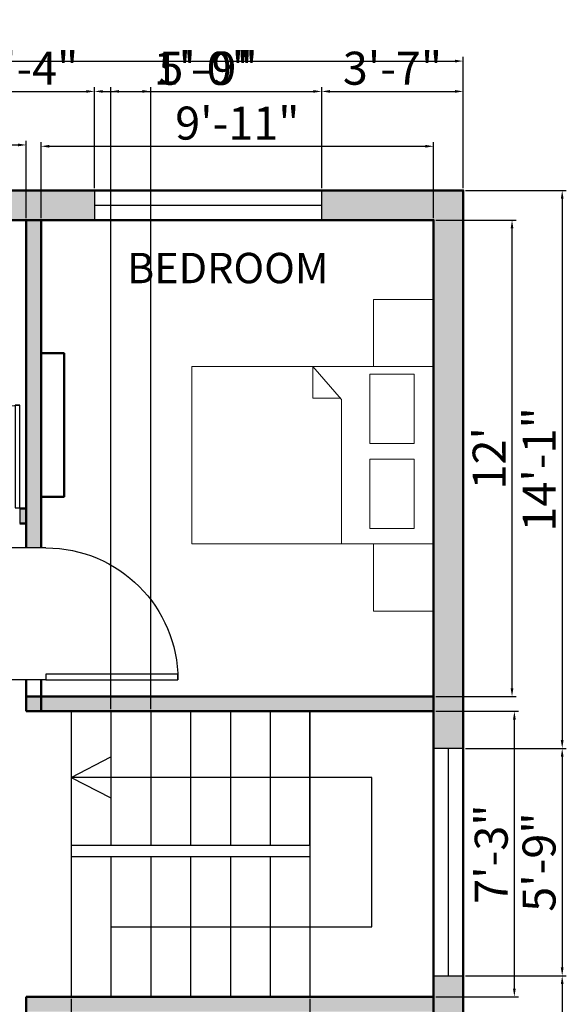
# Model space of a CAD drawing. Units: inches. Extents: x 1344 to 2521, y 3236 to 4924.
# Tile 3 of 14: x 1639 to 1805, y 3517 to 3815. Entities that reach past the tile are written whole.
import ezdxf

# ---------------------------------------------------------------- set-up
doc = ezdxf.new("R2010")
doc.units = ezdxf.units.IN
for name, color, linetype, lineweight in [('A-ANNO-DIMS', 2, 'Continuous', 18), ('A-AREA-IDEN', 3, 'Continuous', 18), ('A-DOOR', 50, 'Continuous', 25), ('A-FLOR-STRS', 7, 'Continuous', 25), ('A-FURN', 130, 'Continuous', 18), ('A-GLAZ', 150, 'Continuous', 25), ('A-WALL', 31, 'Continuous', 50), ('A-WALL-PATT', 8, 'Continuous', 13)]:
    doc.layers.add(name, color=color, linetype=linetype, lineweight=lineweight)
doc.styles.get("Standard").update_dxf_attribs({"font": 'arial.ttf'})
doc.dimstyles.new('ISO-25', dxfattribs={"dimtxt": 10, "dimasz": 2.5, "dimexe": 1.25, "dimexo": 0.625, "dimtad": 1, "dimdec": 0, "dimlunit": 4, "dimtxsty": 'Standard', "dimcen": 2.5, "dimadec": 0, "dimazin": 0, "dimtfac": 1, "dimtdec": 0, "dimtmove": 0, "dimatfit": 3, "dimfxl": 1, "dimarcsym": 0})

# ---------------------------------------------------------------- blocks, each defined once
blk = doc.blocks.new('*U2')
for p, q in [((0, 0), (0, -6)), ((40, 0), (40, -6))]:
    blk.add_line(p, q)
blk.add_lwpolyline([(0, 0), (0, 40), (1.75, 40), (1.75, 0)], close=True)
blk.add_arc((0, 0), 40, 0, 90)
blk = doc.blocks.new('*D32')
at = {"layer": 'A-ANNO-DIMS', "color": 0, "lineweight": -2, "transparency": 16777216}
for p, q in [((1413.52, 3764.06), (1413.52, 3803.88)), ((1773.52, 3764.06), (1773.52, 3803.88)), ((1416.02, 3802.63), (1771.02, 3802.63))]:
    blk.add_line(p, q, dxfattribs=at)
at = {"layer": 'A-ANNO-DIMS', "color": 0, "lineweight": 100, "transparency": 16777216}
for points in [[(1416.02, 3803.04), (1416.02, 3802.21), (1413.52, 3802.63)], [(1771.02, 3803.04), (1771.02, 3802.21), (1773.52, 3802.63)]]:
    blk.add_solid(points, dxfattribs=at)
at = {"layer": 'Defpoints', "color": 0, "lineweight": 100, "transparency": 16777216}
for p in [(1773.52, 3802.63), (1413.52, 3763.43), (1773.52, 3763.43)]:
    blk.add_point(p, dxfattribs=at)
at = {"layer": 'A-ANNO-DIMS', "color": 0, "transparency": 16777216, "insert": (1593.52, 3808.36), "char_height": 10, "attachment_point": 5}
blk.add_mtext("30'", dxfattribs=at)
blk = doc.blocks.new('*D34')
at = {"layer": 'A-ANNO-DIMS', "color": 0, "lineweight": -2, "transparency": 16777216}
for p, q in [((1571.25, 3755.06), (1571.25, 3778.46)), ((1573.75, 3777.21), (1638.44, 3777.21)), ((1640.94, 3755.06), (1640.94, 3778.46))]:
    blk.add_line(p, q, dxfattribs=at)
at = {"layer": 'A-ANNO-DIMS', "color": 0, "lineweight": 100, "transparency": 16777216}
for points in [[(1573.75, 3777.62), (1573.75, 3776.79), (1571.25, 3777.21)], [(1638.44, 3777.62), (1638.44, 3776.79), (1640.94, 3777.21)]]:
    blk.add_solid(points, dxfattribs=at)
at = {"layer": 'Defpoints', "color": 0, "lineweight": 100, "transparency": 16777216}
for p in [(1640.94, 3777.21), (1571.25, 3754.43), (1640.94, 3754.43)]:
    blk.add_point(p, dxfattribs=at)
at = {"layer": 'A-ANNO-DIMS', "color": 0, "transparency": 16777216, "insert": (1606.1, 3782.94), "char_height": 10, "attachment_point": 5}
blk.add_mtext('5\'-10"', dxfattribs=at)
blk = doc.blocks.new('*D35')
at = {"layer": 'A-ANNO-DIMS', "color": 0, "lineweight": -2, "transparency": 16777216}
for p, q in [((1645.44, 3755.06), (1645.44, 3778.05)), ((1647.94, 3776.8), (1762.02, 3776.8)), ((1764.52, 3755.06), (1764.52, 3778.05))]:
    blk.add_line(p, q, dxfattribs=at)
at = {"layer": 'A-ANNO-DIMS', "color": 0, "lineweight": 100, "transparency": 16777216}
for points in [[(1647.94, 3777.22), (1647.94, 3776.38), (1645.44, 3776.8)], [(1762.02, 3777.22), (1762.02, 3776.38), (1764.52, 3776.8)]]:
    blk.add_solid(points, dxfattribs=at)
at = {"layer": 'Defpoints', "color": 0, "lineweight": 100, "transparency": 16777216}
for p in [(1764.52, 3776.8), (1645.44, 3754.43), (1764.52, 3754.43)]:
    blk.add_point(p, dxfattribs=at)
at = {"layer": 'A-ANNO-DIMS', "color": 0, "transparency": 16777216, "insert": (1704.98, 3782.53), "char_height": 10, "attachment_point": 5}
blk.add_mtext('9\'-11"', dxfattribs=at)
blk = doc.blocks.new('*D42')
at = {"layer": 'A-ANNO-DIMS', "color": 0, "lineweight": -2, "transparency": 16777216}
for p, q in [((1765.14, 3605.52), (1790.26, 3605.52)), ((1789.01, 3521.45), (1789.01, 3603.02)), ((1765.14, 3518.95), (1790.26, 3518.95))]:
    blk.add_line(p, q, dxfattribs=at)
at = {"layer": 'A-ANNO-DIMS', "color": 0, "lineweight": 100, "transparency": 16777216}
for points in [[(1788.6, 3603.02), (1789.43, 3603.02), (1789.01, 3605.52)], [(1788.6, 3521.45), (1789.43, 3521.45), (1789.01, 3518.95)]]:
    blk.add_solid(points, dxfattribs=at)
at = {"layer": 'Defpoints', "color": 0, "lineweight": 100, "transparency": 16777216}
for p in [(1764.52, 3605.52), (1789.01, 3605.52), (1764.52, 3518.95)]:
    blk.add_point(p, dxfattribs=at)
at = {"layer": 'A-ANNO-DIMS', "color": 0, "transparency": 16777216, "insert": (1783.28, 3562.24), "char_height": 10, "attachment_point": 5, "rotation": 90}
blk.add_mtext('7\'-3"', dxfattribs=at)
blk = doc.blocks.new('*D43')
at = {"layer": 'A-ANNO-DIMS', "color": 0, "lineweight": -2, "transparency": 16777216}
for p, q in [((1765.14, 3754.43), (1789.55, 3754.43)), ((1788.3, 3612.52), (1788.3, 3751.93)), ((1765.14, 3610.02), (1789.55, 3610.02))]:
    blk.add_line(p, q, dxfattribs=at)
at = {"layer": 'A-ANNO-DIMS', "color": 0, "lineweight": 100, "transparency": 16777216}
for points in [[(1787.88, 3751.93), (1788.72, 3751.93), (1788.3, 3754.43)], [(1787.88, 3612.52), (1788.72, 3612.52), (1788.3, 3610.02)]]:
    blk.add_solid(points, dxfattribs=at)
at = {"layer": 'Defpoints', "color": 0, "lineweight": 100, "transparency": 16777216}
for p in [(1764.52, 3754.43), (1788.3, 3754.43), (1764.52, 3610.02)]:
    blk.add_point(p, dxfattribs=at)
at = {"layer": 'A-ANNO-DIMS', "color": 0, "transparency": 16777216, "insert": (1782.66, 3682.23), "char_height": 10, "attachment_point": 5, "rotation": 90}
blk.add_mtext("12'", dxfattribs=at)
blk = doc.blocks.new('BED-DOUBLE')
for p, q in [((27.95, 53.78), (27.95, 9.98)), ((27.95, 9.98), (36.68, 0)), ((36.68, 9.56), (28.32, 9.56)), ((36.68, 0), (36.68, 9.56))]:
    blk.add_line(p, q)
for points in [[(0, 0), (73.35, 0), (73.35, 53.78), (0, 53.78)], [(5.91, 28.08), (19.39, 28.08), (19.39, 49.13), (5.91, 49.13)], [(5.91, 2.27), (19.39, 2.27), (19.39, 23.31), (5.91, 23.31)]]:
    blk.add_lwpolyline(points, close=True)
blk = doc.blocks.new('*D159')
at = {"layer": 'A-ANNO-DIMS', "color": 0, "lineweight": -2, "transparency": 16777216}
for p, q in [((1621.71, 3764.06), (1621.71, 3794.68)), ((1661.64, 3764.06), (1661.64, 3794.68)), ((1624.21, 3793.43), (1659.14, 3793.43))]:
    blk.add_line(p, q, dxfattribs=at)
at = {"layer": 'A-ANNO-DIMS', "color": 0, "lineweight": 100, "transparency": 16777216}
for points in [[(1624.21, 3793.85), (1624.21, 3793.02), (1621.71, 3793.43)], [(1659.14, 3793.85), (1659.14, 3793.02), (1661.64, 3793.43)]]:
    blk.add_solid(points, dxfattribs=at)
at = {"layer": 'Defpoints', "color": 0, "lineweight": 100, "transparency": 16777216}
for p in [(1661.64, 3793.43), (1621.71, 3763.43), (1661.64, 3763.43)]:
    blk.add_point(p, dxfattribs=at)
at = {"layer": 'A-ANNO-DIMS', "color": 0, "transparency": 16777216, "insert": (1641.68, 3799.17), "char_height": 10, "attachment_point": 5}
blk.add_mtext('3\'-4"', dxfattribs=at)
blk = doc.blocks.new('*D160')
at = {"layer": 'A-ANNO-DIMS', "color": 0, "lineweight": -2, "transparency": 16777216}
for p, q in [((1661.64, 3764.06), (1661.64, 3794.68)), ((1730.56, 3764.06), (1730.56, 3794.68)), ((1664.14, 3793.43), (1728.06, 3793.43))]:
    blk.add_line(p, q, dxfattribs=at)
at = {"layer": 'A-ANNO-DIMS', "color": 0, "lineweight": 100, "transparency": 16777216}
for points in [[(1664.14, 3793.85), (1664.14, 3793.02), (1661.64, 3793.43)], [(1728.06, 3793.85), (1728.06, 3793.02), (1730.56, 3793.43)]]:
    blk.add_solid(points, dxfattribs=at)
at = {"layer": 'Defpoints', "color": 0, "lineweight": 100, "transparency": 16777216}
for p in [(1730.56, 3793.43), (1661.64, 3763.43), (1730.56, 3763.43)]:
    blk.add_point(p, dxfattribs=at)
at = {"layer": 'A-ANNO-DIMS', "color": 0, "transparency": 16777216, "insert": (1696.1, 3799.16), "char_height": 10, "attachment_point": 5}
blk.add_mtext('5\'-9"', dxfattribs=at)
blk = doc.blocks.new('*D161')
at = {"layer": 'A-ANNO-DIMS', "color": 0, "lineweight": -2, "transparency": 16777216}
for p, q in [((1730.56, 3764.06), (1730.56, 3794.68)), ((1773.52, 3764.06), (1773.52, 3794.68)), ((1733.06, 3793.43), (1771.02, 3793.43))]:
    blk.add_line(p, q, dxfattribs=at)
at = {"layer": 'A-ANNO-DIMS', "color": 0, "lineweight": 100, "transparency": 16777216}
for points in [[(1733.06, 3793.85), (1733.06, 3793.02), (1730.56, 3793.43)], [(1771.02, 3793.85), (1771.02, 3793.02), (1773.52, 3793.43)]]:
    blk.add_solid(points, dxfattribs=at)
at = {"layer": 'Defpoints', "color": 0, "lineweight": 100, "transparency": 16777216}
for p in [(1773.52, 3793.43), (1730.56, 3763.43), (1773.52, 3763.43)]:
    blk.add_point(p, dxfattribs=at)
at = {"layer": 'A-ANNO-DIMS', "color": 0, "transparency": 16777216, "insert": (1752.04, 3799.17), "char_height": 10, "attachment_point": 5}
blk.add_mtext('3\'-7"', dxfattribs=at)
blk = doc.blocks.new('*D169')
at = {"layer": 'A-ANNO-DIMS', "color": 0, "lineweight": -2, "transparency": 16777216}
for p, q in [((1774.14, 3763.43), (1804.77, 3763.43)), ((1803.52, 3760.93), (1803.52, 3596.78)), ((1774.14, 3594.28), (1804.77, 3594.28))]:
    blk.add_line(p, q, dxfattribs=at)
at = {"layer": 'A-ANNO-DIMS', "color": 0, "lineweight": 100, "transparency": 16777216}
for points in [[(1803.1, 3760.93), (1803.93, 3760.93), (1803.52, 3763.43)], [(1803.1, 3596.78), (1803.93, 3596.78), (1803.52, 3594.28)]]:
    blk.add_solid(points, dxfattribs=at)
at = {"layer": 'Defpoints', "color": 0, "lineweight": 100, "transparency": 16777216}
for p in [(1773.52, 3763.43), (1773.52, 3594.28), (1803.52, 3594.28)]:
    blk.add_point(p, dxfattribs=at)
at = {"layer": 'A-ANNO-DIMS', "color": 0, "transparency": 16777216, "insert": (1797.87, 3678.86), "char_height": 10, "attachment_point": 5, "rotation": 90}
blk.add_mtext('14\'-1"', dxfattribs=at)
blk = doc.blocks.new('*D170')
at = {"layer": 'A-ANNO-DIMS', "color": 0, "lineweight": -2, "transparency": 16777216}
for p, q in [((1774.14, 3594.28), (1804.77, 3594.28)), ((1803.52, 3591.78), (1803.52, 3527.86)), ((1774.14, 3525.36), (1804.77, 3525.36))]:
    blk.add_line(p, q, dxfattribs=at)
at = {"layer": 'A-ANNO-DIMS', "color": 0, "lineweight": 100, "transparency": 16777216}
for points in [[(1803.1, 3591.78), (1803.93, 3591.78), (1803.52, 3594.28)], [(1803.1, 3527.86), (1803.93, 3527.86), (1803.52, 3525.36)]]:
    blk.add_solid(points, dxfattribs=at)
at = {"layer": 'Defpoints', "color": 0, "lineweight": 100, "transparency": 16777216}
for p in [(1773.52, 3594.28), (1773.52, 3525.36), (1803.52, 3525.36)]:
    blk.add_point(p, dxfattribs=at)
at = {"layer": 'A-ANNO-DIMS', "color": 0, "transparency": 16777216, "insert": (1797.79, 3559.82), "char_height": 10, "attachment_point": 5, "rotation": 90}
blk.add_mtext('5\'-9"', dxfattribs=at)
blk = doc.blocks.new('*D171')
at = {"layer": 'A-ANNO-DIMS', "color": 0, "lineweight": -2, "transparency": 16777216}
for p, q in [((1774.14, 3525.36), (1804.77, 3525.36)), ((1803.52, 3522.86), (1803.52, 3350.01)), ((1774.14, 3347.51), (1804.77, 3347.51))]:
    blk.add_line(p, q, dxfattribs=at)
at = {"layer": 'A-ANNO-DIMS', "color": 0, "lineweight": 100, "transparency": 16777216}
for points in [[(1803.1, 3522.86), (1803.93, 3522.86), (1803.52, 3525.36)], [(1803.1, 3350.01), (1803.93, 3350.01), (1803.52, 3347.51)]]:
    blk.add_solid(points, dxfattribs=at)
at = {"layer": 'Defpoints', "color": 0, "lineweight": 100, "transparency": 16777216}
for p in [(1773.52, 3525.36), (1773.52, 3347.51), (1803.52, 3347.51)]:
    blk.add_point(p, dxfattribs=at)
at = {"layer": 'A-ANNO-DIMS', "color": 0, "transparency": 16777216, "insert": (1797.79, 3436.44), "char_height": 10, "attachment_point": 5, "rotation": 90}
blk.add_mtext('14\'-10"', dxfattribs=at)
blk = doc.blocks.new('*D180')
at = {"layer": 'A-ANNO-DIMS', "color": 0, "lineweight": -2, "transparency": 16777216}
for p, q in [((1644.82, 3655.04), (1382.27, 3655.04)), ((1383.52, 3652.54), (1383.52, 3617.54)), ((1644.82, 3615.04), (1382.27, 3615.04))]:
    blk.add_line(p, q, dxfattribs=at)
at = {"layer": 'A-ANNO-DIMS', "color": 0, "lineweight": 100, "transparency": 16777216}
for points in [[(1383.1, 3652.54), (1383.93, 3652.54), (1383.52, 3655.04)], [(1383.1, 3617.54), (1383.93, 3617.54), (1383.52, 3615.04)]]:
    blk.add_solid(points, dxfattribs=at)
at = {"layer": 'Defpoints', "color": 0, "lineweight": 100, "transparency": 16777216}
for p in [(1645.44, 3655.04), (1383.52, 3615.04), (1645.44, 3615.04)]:
    blk.add_point(p, dxfattribs=at)
at = {"layer": 'A-ANNO-DIMS', "color": 0, "transparency": 16777216, "insert": (1377.78, 3635.04), "char_height": 10, "attachment_point": 5, "rotation": 90}
blk.add_mtext('3\'-4"', dxfattribs=at)
blk = doc.blocks.new('*D184')
at = {"layer": 'A-ANNO-DIMS', "color": 0, "lineweight": -2, "transparency": 16777216}
for p, q in [((1654.54, 3518.32), (1654.54, 3316.22)), ((1727.01, 3518.32), (1727.01, 3316.22)), ((1657.04, 3317.47), (1724.51, 3317.47))]:
    blk.add_line(p, q, dxfattribs=at)
at = {"layer": 'A-ANNO-DIMS', "color": 0, "lineweight": 100, "transparency": 16777216}
for points in [[(1657.04, 3317.89), (1657.04, 3317.06), (1654.54, 3317.47)], [(1724.51, 3317.89), (1724.51, 3317.06), (1727.01, 3317.47)]]:
    blk.add_solid(points, dxfattribs=at)
at = {"layer": 'Defpoints', "color": 0, "lineweight": 100, "transparency": 16777216}
for p in [(1654.54, 3518.95), (1727.01, 3518.95), (1727.01, 3317.47)]:
    blk.add_point(p, dxfattribs=at)
at = {"layer": 'A-ANNO-DIMS', "color": 0, "transparency": 16777216, "insert": (1690.78, 3323.27), "char_height": 10, "attachment_point": 5}
blk.add_mtext('6\'-0 1/2"', dxfattribs=at)
blk = doc.blocks.new('*D185')
at = {"layer": 'A-ANNO-DIMS', "color": 0, "lineweight": -2, "transparency": 16777216}
for p, q in [((1666.62, 3606.15), (1666.62, 3794.68)), ((1678.7, 3606.15), (1678.7, 3794.68)), ((1669.12, 3793.43), (1676.2, 3793.43)), ((1678.7, 3793.43), (1708.09, 3793.43))]:
    blk.add_line(p, q, dxfattribs=at)
at = {"layer": 'A-ANNO-DIMS', "color": 0, "lineweight": 100, "transparency": 16777216}
for points in [[(1669.12, 3793.85), (1669.12, 3793.02), (1666.62, 3793.43)], [(1676.2, 3793.85), (1676.2, 3793.02), (1678.7, 3793.43)]]:
    blk.add_solid(points, dxfattribs=at)
at = {"layer": 'Defpoints', "color": 0, "lineweight": 100, "transparency": 16777216}
for p in [(1678.7, 3793.43), (1666.62, 3605.52), (1678.7, 3605.52)]:
    blk.add_point(p, dxfattribs=at)
at = {"layer": 'A-ANNO-DIMS', "color": 0, "transparency": 16777216, "insert": (1694.64, 3799.16), "char_height": 10, "attachment_point": 5}
blk.add_mtext('1\'-0"', dxfattribs=at)

msp = doc.modelspace()

# ---------------------------------------------------------------- hatches: boundary and pattern name
at = {"layer": 'A-WALL-PATT'}
h = msp.add_hatch(color=256, dxfattribs=at)
h.dxf.hatch_style = 1
h.paths.add_polyline_path([(1452.8, 3763.43), (1413.52, 3763.43), (1413.52, 3608.87), (1422.52, 3608.87), (1422.52, 3754.43), (1452.8, 3754.43)])
h.paths.add_polyline_path([(1588.61, 3763.43), (1521.72, 3763.43), (1521.72, 3754.43), (1588.61, 3754.43)])
h.paths.add_polyline_path([(1661.64, 3763.43), (1621.71, 3763.43), (1621.71, 3754.43), (1661.64, 3754.43)])
h.paths.add_polyline_path([(1773.52, 3763.43), (1730.56, 3763.43), (1730.56, 3754.43), (1764.52, 3754.43), (1764.52, 3594.28), (1773.52, 3594.28)])
h.paths.add_polyline_path([(1645.44, 3754.43), (1640.94, 3754.43), (1640.94, 3655.04), (1645.44, 3655.04)])
h.paths.add_polyline_path([(1571.25, 3754.43), (1566.75, 3754.43), (1566.75, 3624.19), (1566.51, 3624.19), (1564.17, 3624.19), (1564.17, 3619.69), (1571.25, 3619.69)])
h.paths.add_polyline_path([(1607.83, 3666.99), (1571.25, 3666.99), (1571.25, 3662.49), (1607.83, 3662.49)])
h.paths.add_polyline_path([(1640.94, 3666.99), (1638.96, 3666.99), (1638.96, 3662.49), (1640.94, 3662.49)])
h.paths.add_polyline_path([(1524.17, 3624.19), (1517.67, 3624.19), (1517.67, 3619.69), (1524.17, 3619.69)])
h = msp.add_hatch(color=256, dxfattribs=at)
h.dxf.hatch_style = 1
h.paths.add_polyline_path([(1451.85, 3356.47), (1422.52, 3356.47), (1422.52, 3386.9), (1413.52, 3386.9), (1413.52, 3347.51), (1451.85, 3347.51)])
h.paths.add_polyline_path([(1744.16, 3352.01), (1566.75, 3352.01), (1566.75, 3356.47), (1544.82, 3356.47), (1520.77, 3356.47), (1520.77, 3347.51), (1744.16, 3347.51)])
h.paths.add_polyline_path([(1773.52, 3525.36), (1764.52, 3525.36), (1764.52, 3497.27), (1764.52, 3412.01), (1764.72, 3412.01), (1764.72, 3403.01), (1764.52, 3403.01), (1764.52, 3356.51), (1744.16, 3356.51), (1744.16, 3347.51), (1773.52, 3347.51)])
h.paths.add_polyline_path([(1764.52, 3412.01), (1740.62, 3412.01), (1740.62, 3403.01), (1764.52, 3403.01)])
h.paths.add_polyline_path([(1668.63, 3412.01), (1644.53, 3412.01), (1644.53, 3403.01), (1668.63, 3403.01)])
h.paths.add_polyline_path([(1571.25, 3514.45), (1571.25, 3518.95), (1564.17, 3518.95), (1564.17, 3514.45), (1566.75, 3514.45), (1566.75, 3352.01), (1571.25, 3352.01)])
h.paths.add_polyline_path([(1422.52, 3527.47), (1413.52, 3527.47), (1413.52, 3455.82), (1422.52, 3455.82), (1422.52, 3470.24)])
h.paths.add_polyline_path([(1488.21, 3517.8, -0.012876), (1488.24, 3518.95), (1422.52, 3518.95), (1422.52, 3514.45), (1488.21, 3514.45)])
h.paths.add_polyline_path([(1524.17, 3518.95), (1510.55, 3518.95), (1510.55, 3517.8), (1510.55, 3514.45), (1524.17, 3514.45)])
h.paths.add_polyline_path([(1764.52, 3518.95), (1640.94, 3518.95), (1640.94, 3514.45), (1764.52, 3514.45)])
h.paths.add_polyline_path([(1764.52, 3610.02), (1645.44, 3610.02), (1645.44, 3605.52), (1764.52, 3605.52)])
h.paths.add_polyline_path([(1645.44, 3610.02), (1640.94, 3610.02), (1640.94, 3605.52), (1645.44, 3605.52)])
h.paths.add_polyline_path([(1422.52, 3580.89), (1413.52, 3580.89), (1413.52, 3555.45), (1422.52, 3555.45)])
h.paths.add_polyline_path([(1513.17, 3573.32), (1505.17, 3573.32), (1505.17, 3573.28), (1475.67, 3573.28), (1422.52, 3573.32), (1422.52, 3568.82), (1513.17, 3568.82)])
h.paths.add_polyline_path([(1635.28, 3376.69), (1701.38, 3376.69), (1701.38, 3395.67), (1635.28, 3395.67)], flags=9)
h.paths.add_polyline_path([(1526.07, 3560.64), (1635.07, 3560.64), (1635.07, 3579.62), (1526.07, 3579.62)], flags=9)
h.paths.add_polyline_path([(1666.39, 3730.09), (1741.06, 3730.09), (1741.06, 3749.07), (1666.39, 3749.07)], flags=9)
h.paths.add_polyline_path([(1446.44, 3467.76), (1517.54, 3467.76), (1517.54, 3502.26), (1446.44, 3502.26)], flags=9)
h.paths.add_polyline_path([(1429.07, 3520.24), (1478.72, 3520.24), (1478.72, 3539.22), (1429.07, 3539.22)], flags=9)
h.paths.add_polyline_path([(1425.85, 3603.57), (1475.5, 3603.57), (1475.5, 3622.55), (1425.85, 3622.55)], flags=9)
h.paths.add_polyline_path([(1570.93, 3699.42), (1620.58, 3699.42), (1620.58, 3718.41), (1570.93, 3718.41)], flags=9)
h.paths.add_polyline_path([(1447.04, 3718.72), (1518.14, 3718.72), (1518.14, 3753.22), (1447.04, 3753.22)], flags=9)

# ---------------------------------------------------------------- linework, layer by layer
at = {"layer": 'A-FLOR-STRS'}
for p, q in [((1654.54, 3605.52), (1654.54, 3518.95)), ((1666.62, 3605.52), (1666.62, 3564.91)), ((1678.7, 3605.52), (1678.7, 3564.91)), ((1690.78, 3605.52), (1690.78, 3564.91)), ((1702.86, 3605.52), (1702.86, 3564.91)), ((1714.94, 3605.52), (1714.94, 3564.91)), ((1727.01, 3564.91), (1727.01, 3605.52)), ((1727.01, 3605.52), (1727.01, 3518.95)), ((1654.54, 3585.5), (1666.62, 3591.67)), ((1745.79, 3585.5), (1654.54, 3585.5)), ((1654.54, 3585.5), (1666.62, 3579.32)), ((1745.79, 3540.2), (1745.79, 3585.5)), ((1666.62, 3561.45), (1666.62, 3518.95)), ((1678.7, 3561.45), (1678.7, 3518.95)), ((1690.78, 3561.45), (1690.78, 3518.95)), ((1702.86, 3561.45), (1702.86, 3518.95)), ((1714.94, 3561.45), (1714.94, 3518.95)), ((1666.62, 3540.2), (1745.79, 3540.2))]:
    msp.add_line(p, q, dxfattribs=at)
msp.add_lwpolyline([(1654.54, 3564.91), (1727.01, 3564.91), (1727.01, 3561.45), (1654.54, 3561.45)], dxfattribs=at)
at = {"layer": 'A-FURN'}
for points in [[(1764.52, 3730.36), (1746.29, 3730.36), (1746.29, 3710.02), (1764.52, 3710.02)], [(1764.52, 3656.24), (1746.29, 3656.24), (1746.29, 3635.89), (1764.52, 3635.89)]]:
    msp.add_lwpolyline(points, close=True, dxfattribs=at)
at = {"layer": 'A-GLAZ'}
for p, q in [((1661.64, 3758.93), (1730.56, 3758.93)), ((1769.02, 3525.36), (1769.02, 3594.28))]:
    msp.add_line(p, q, dxfattribs=at)
for points in [[(1661.64, 3763.43), (1661.64, 3754.43), (1730.56, 3754.43), (1730.56, 3763.43)], [(1764.52, 3525.36), (1773.52, 3525.36), (1773.52, 3594.28), (1764.52, 3594.28)]]:
    msp.add_lwpolyline(points, close=True, dxfattribs=at)
at = {"layer": 'A-WALL'}
for p, q in [((1640.94, 3655.04), (1640.94, 3754.43)), ((1645.44, 3655.04), (1645.44, 3754.43)), ((1640.94, 3735.69), (1640.94, 3655.04)), ((1645.44, 3735.69), (1645.44, 3655.04)), ((1638.96, 3666.99), (1640.94, 3666.99)), ((1638.96, 3662.49), (1640.94, 3662.49)), ((1640.94, 3605.52), (1640.94, 3615.04)), ((1640.94, 3615.04), (1640.94, 3605.52)), ((1645.44, 3605.52), (1645.44, 3615.04)), ((1645.44, 3615.04), (1645.44, 3605.52)), ((1764.52, 3610.02), (1640.94, 3610.02)), ((1764.52, 3605.52), (1640.94, 3605.52)), ((1764.52, 3533.27), (1764.52, 3497.27)), ((1640.94, 3518.95), (1764.52, 3518.95)), ((1640.94, 3518.95), (1640.94, 3514.45))]:
    msp.add_line(p, q, dxfattribs=at)
for points in [[(1773.52, 3347.51), (1773.52, 3763.43), (1413.52, 3763.43), (1413.52, 3347.51)], [(1764.52, 3356.51), (1764.52, 3754.43), (1422.52, 3754.43), (1422.52, 3356.47)]]:
    msp.add_lwpolyline(points, dxfattribs=at)
msp.add_lwpolyline([(1645.44, 3670.57), (1652.42, 3670.57), (1652.42, 3714.04), (1645.44, 3714.04)], close=True, dxfattribs=at)

# ---------------------------------------------------------------- block references
at = {"layer": 'A-DOOR', "xscale": -0.7782718260199863, "yscale": 0.7782718260199863, "zscale": 0.7782718260199863}
msp.add_blockref('*U2', (1638.96, 3667.16), dxfattribs=at)
at = {"layer": 'A-DOOR', "xscale": -1, "rotation": 270}
msp.add_blockref('*U2', (1646.94, 3615.04), dxfattribs=at)
at = {"layer": 'A-FURN', "rotation": 180}
msp.add_blockref('BED-DOUBLE', (1764.52, 3710.02), dxfattribs=at)

# ---------------------------------------------------------------- texts
at = {"layer": 'A-AREA-IDEN', "insert": (1668.7, 3744.5), "char_height": 9.211, "attachment_point": 1}
msp.add_mtext_dynamic_manual_height_columns(' BEDROOM', width=108.7809, gutter_width=46.06, heights=[0], dxfattribs=at)

# ---------------------------------------------------------------- dimensions: what is measured, and where the dimension line sits
at = {"layer": 'A-ANNO-DIMS'}
for base, p1, p2, override, picture, middle in [((1773.52, 3802.63), (1413.52, 3763.43), (1773.52, 3763.43), {"dimclrd": 0, "dimclre": 0, "dimclrt": 0}, '*D32', (1593.52, 3808.36)), ((1661.64, 3793.43), (1621.71, 3763.43), (1661.64, 3763.43), {"dimdec": 1, "dimlfac": 1, "dimrnd": 0, "dimzin": 1, "dimdsep": 46, "dimlunit": 4, "dimfrac": 2}, '*D159', (1641.68, 3799.17)), ((1730.56, 3793.43), (1661.64, 3763.43), (1730.56, 3763.43), {"dimdec": 1, "dimlfac": 1, "dimrnd": 0, "dimzin": 1, "dimdsep": 46, "dimlunit": 4, "dimfrac": 2}, '*D160', (1696.1, 3799.16)), ((1678.7, 3793.43), (1666.62, 3605.52), (1678.7, 3605.52), {"dimdec": 1, "dimlfac": 1, "dimrnd": 0, "dimzin": 1, "dimdsep": 46, "dimlunit": 4, "dimfrac": 2}, '*D185', (1694.64, 3799.16)), ((1773.52, 3793.43), (1730.56, 3763.43), (1773.52, 3763.43), {"dimdec": 1, "dimlfac": 1, "dimrnd": 0, "dimzin": 1, "dimdsep": 46, "dimlunit": 4, "dimfrac": 2}, '*D161', (1752.04, 3799.17)), ((1640.94, 3777.21), (1571.25, 3754.43), (1640.94, 3754.43), {"dimclrd": 0, "dimclre": 0, "dimclrt": 0}, '*D34', (1606.1, 3782.94)), ((1764.52, 3776.8), (1645.44, 3754.43), (1764.52, 3754.43), {"dimclrd": 0, "dimclre": 0, "dimclrt": 0}, '*D35', (1704.98, 3782.53)), ((1727.01, 3317.47), (1654.54, 3518.95), (1727.01, 3518.95), {"dimdec": 1, "dimlfac": 1, "dimrnd": 0, "dimzin": 1, "dimdsep": 46, "dimlunit": 4, "dimfrac": 2}, '*D184', (1690.78, 3323.27))]:
    dim = msp.add_linear_dim(base=base, p1=p1, p2=p2, dimstyle='ISO-25', override=override, dxfattribs=at)
    dim.commit()
    dim.dimension.update_dxf_attribs({"geometry": picture, "text_midpoint": middle})
for base, p1, p2, override, picture, middle in [((1803.5178, 3594.2838), (1773.5178, 3763.4321), (1773.5178, 3594.2838), {"dimdec": 1, "dimlfac": 1, "dimrnd": 0, "dimzin": 1, "dimdsep": 46, "dimlunit": 4, "dimfrac": 2}, '*D169', (1797.8723, 3678.858)), ((1788.3, 3754.43), (1764.52, 3610.02), (1764.52, 3754.43), {"dimclrd": 0, "dimclre": 0, "dimclrt": 0}, '*D43', (1782.66, 3682.23)), ((1383.52, 3615.04), (1645.44, 3655.04), (1645.44, 3615.04), {"dimdec": 1, "dimlfac": 1, "dimrnd": 0, "dimzin": 1, "dimdsep": 46, "dimlunit": 4, "dimfrac": 2}, '*D180', (1377.78, 3635.04)), ((1789.01, 3605.52), (1764.52, 3518.95), (1764.52, 3605.52), {"dimclrd": 0, "dimclre": 0, "dimclrt": 0}, '*D42', (1783.28, 3562.24)), ((1803.52, 3525.36), (1773.52, 3594.28), (1773.52, 3525.36), {"dimdec": 1, "dimlfac": 1, "dimrnd": 0, "dimzin": 1, "dimdsep": 46, "dimlunit": 4, "dimfrac": 2}, '*D170', (1797.79, 3559.82)), ((1803.5178, 3347.5114), (1773.5178, 3525.3602), (1773.5178, 3347.5114), {"dimdec": 1, "dimlfac": 1, "dimrnd": 0, "dimzin": 1, "dimdsep": 46, "dimlunit": 4, "dimfrac": 2}, '*D171', (1797.7871, 3436.4358))]:
    dim = msp.add_linear_dim(base=base, p1=p1, p2=p2, angle=90, dimstyle='ISO-25', override=override, dxfattribs=at)
    dim.commit()
    dim.dimension.update_dxf_attribs({"geometry": picture, "text_midpoint": middle})

doc.saveas('drawing.dxf')
